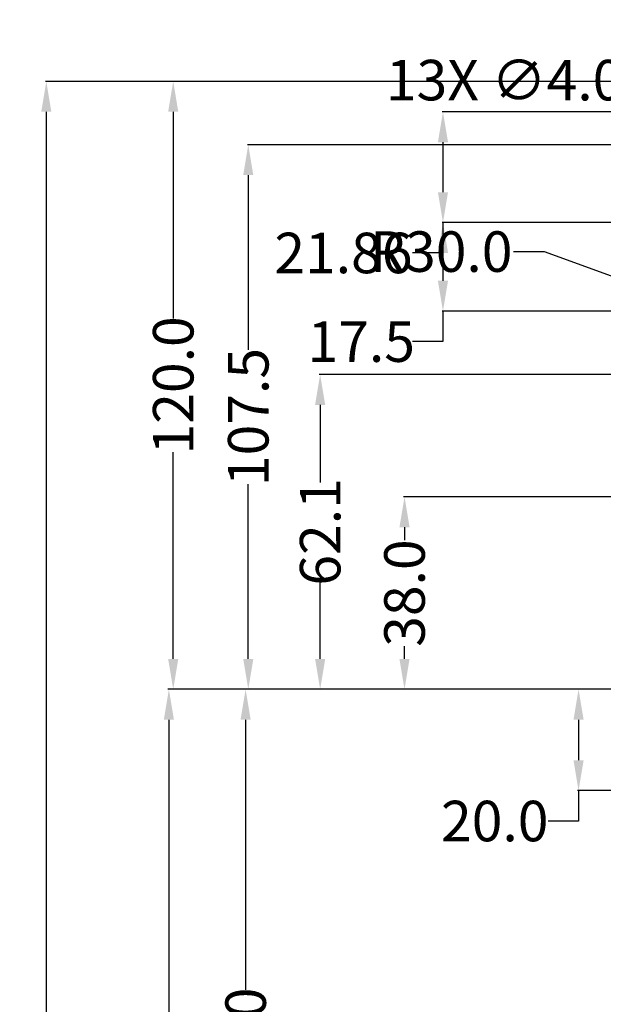
# Model space of a CAD drawing. Units: inches. Extents: x 11765 to 12471, y 10149 to 10793.
# Tile 3 of 8: x 11765 to 11880, y 10530 to 10724. Entities that reach past the tile are written whole.
import ezdxf

# ---------------------------------------------------------------- set-up
doc = ezdxf.new("R2010")
doc.units = ezdxf.units.IN
doc.header["$MEASUREMENT"] = 0
doc.layers.add('M-DIMS', color=2, linetype='Continuous', lineweight=25)
doc.styles.get("Standard").update_dxf_attribs({"font": 'arial.ttf'})
doc.dimstyles.get("Standard").update_dxf_attribs({"dimtxt": 8, "dimasz": 6, "dimexe": 0.18, "dimexo": 0.0625, "dimgap": 0.09, "dimtad": 0, "dimtoh": 1, "dimdec": 1, "dimzin": 0, "dimdsep": 46, "dimtxsty": 'Standard', "dimcen": 0.09, "dimadec": 0, "dimazin": 0, "dimtfac": 1, "dimtdec": 1, "dimtofl": 0, "dimtmove": 0, "dimatfit": 3, "dimfxl": 1, "dimtolj": 1, "dimtzin": 0, "dimarcsym": 0})

# ---------------------------------------------------------------- blocks, each defined once
blk = doc.blocks.new('*D6')
at = {"layer": 'Defpoints', "color": 0, "transparency": 16777216}
for p in [(11882.91, 10712.15), (11769.87, 10237.15), (11917.55, 10237.15)]:
    blk.add_point(p, dxfattribs=at)
at = {"layer": 'M-DIMS', "color": 0, "lineweight": -2, "transparency": 16777216}
for p, q in [((11882.85, 10712.15), (11769.69, 10712.15)), ((11769.87, 10706.15), (11769.87, 10488.38)), ((11769.87, 10243.15), (11769.87, 10460.91)), ((11917.49, 10237.15), (11769.69, 10237.15))]:
    blk.add_line(p, q, dxfattribs=at)
at = {"layer": 'M-DIMS', "color": 0, "transparency": 16777216}
for points in [[(11768.87, 10706.15), (11770.87, 10706.15), (11769.87, 10712.15)], [(11768.87, 10243.15), (11770.87, 10243.15), (11769.87, 10237.15)]]:
    blk.add_solid(points, dxfattribs=at)
at = {"layer": 'M-DIMS', "color": 0, "transparency": 16777216, "insert": (11769.87, 10474.65), "char_height": 8, "attachment_point": 5, "rotation": 90}
blk.add_mtext('\\A1;475.0', dxfattribs=at)
blk = doc.blocks.new('*D24')
at = {"layer": 'Defpoints', "color": 0, "transparency": 16777216}
for p in [(11794.92, 10712.15), (11882.91, 10712.15), (11882.91, 10592.15)]:
    blk.add_point(p, dxfattribs=at)
at = {"layer": 'M-DIMS', "color": 0, "lineweight": -2, "transparency": 16777216}
for p, q in [((11882.85, 10712.15), (11794.74, 10712.15)), ((11794.92, 10706.15), (11794.92, 10665.34)), ((11794.92, 10598.15), (11794.92, 10638.95)), ((11882.85, 10592.15), (11794.74, 10592.15))]:
    blk.add_line(p, q, dxfattribs=at)
at = {"layer": 'M-DIMS', "color": 0, "transparency": 16777216}
for points in [[(11793.92, 10706.15), (11795.92, 10706.15), (11794.92, 10712.15)], [(11793.92, 10598.15), (11795.92, 10598.15), (11794.92, 10592.15)]]:
    blk.add_solid(points, dxfattribs=at)
at = {"layer": 'M-DIMS', "color": 0, "transparency": 16777216, "insert": (11794.92, 10652.15), "char_height": 8, "attachment_point": 5, "rotation": 90}
blk.add_mtext('\\A1;120.0', dxfattribs=at)
blk = doc.blocks.new('*D25')
at = {"layer": 'Defpoints', "color": 0, "transparency": 16777216}
for p in [(11894.91, 10699.65), (11809.73, 10592.15), (11882.91, 10592.15)]:
    blk.add_point(p, dxfattribs=at)
at = {"layer": 'M-DIMS', "color": 0, "lineweight": -2, "transparency": 16777216}
for p, q in [((11894.85, 10699.65), (11809.55, 10699.65)), ((11809.73, 10693.65), (11809.73, 10659.14)), ((11809.73, 10598.15), (11809.73, 10632.65)), ((11882.85, 10592.15), (11809.55, 10592.15))]:
    blk.add_line(p, q, dxfattribs=at)
at = {"layer": 'M-DIMS', "color": 0, "transparency": 16777216}
for points in [[(11808.73, 10693.65), (11810.73, 10693.65), (11809.73, 10699.65)], [(11808.73, 10598.15), (11810.73, 10598.15), (11809.73, 10592.15)]]:
    blk.add_solid(points, dxfattribs=at)
at = {"layer": 'M-DIMS', "color": 0, "transparency": 16777216, "insert": (11809.73, 10645.9), "char_height": 8, "attachment_point": 5, "rotation": 90}
blk.add_mtext('\\A1;107.5', dxfattribs=at)
blk = doc.blocks.new('*D26')
at = {"layer": 'Defpoints', "color": 0, "transparency": 16777216}
for p in [(11934.91, 10654.29), (11823.92, 10592.15), (11882.91, 10592.15)]:
    blk.add_point(p, dxfattribs=at)
at = {"layer": 'M-DIMS', "color": 0, "lineweight": -2, "transparency": 16777216}
for p, q in [((11934.85, 10654.29), (11823.74, 10654.29)), ((11823.92, 10648.29), (11823.92, 10632.95)), ((11823.92, 10598.15), (11823.92, 10613.49)), ((11882.85, 10592.15), (11823.74, 10592.15))]:
    blk.add_line(p, q, dxfattribs=at)
at = {"layer": 'M-DIMS', "color": 0, "transparency": 16777216}
for points in [[(11822.92, 10648.29), (11824.92, 10648.29), (11823.92, 10654.29)], [(11822.92, 10598.15), (11824.92, 10598.15), (11823.92, 10592.15)]]:
    blk.add_solid(points, dxfattribs=at)
at = {"layer": 'M-DIMS', "color": 0, "transparency": 16777216, "insert": (11823.92, 10623.22), "char_height": 8, "attachment_point": 5, "rotation": 90}
blk.add_mtext('\\A1;62.1', dxfattribs=at)
blk = doc.blocks.new('*D27')
at = {"layer": 'Defpoints', "color": 0, "transparency": 16777216}
for p in [(11840.57, 10630.15), (11942.91, 10630.15), (11942.91, 10592.15)]:
    blk.add_point(p, dxfattribs=at)
at = {"layer": 'M-DIMS', "color": 0, "lineweight": -2, "transparency": 16777216}
for p, q in [((11942.85, 10630.15), (11840.39, 10630.15)), ((11840.57, 10624.15), (11840.57, 10621.61)), ((11840.57, 10598.15), (11840.57, 10600.68)), ((11942.85, 10592.15), (11840.39, 10592.15))]:
    blk.add_line(p, q, dxfattribs=at)
at = {"layer": 'M-DIMS', "color": 0, "transparency": 16777216}
for points in [[(11839.57, 10624.15), (11841.57, 10624.15), (11840.57, 10630.15)], [(11839.57, 10598.15), (11841.57, 10598.15), (11840.57, 10592.15)]]:
    blk.add_solid(points, dxfattribs=at)
at = {"layer": 'M-DIMS', "color": 0, "transparency": 16777216, "insert": (11840.57, 10611.15), "char_height": 8, "attachment_point": 5, "rotation": 90}
blk.add_mtext('\\A1;38.0', dxfattribs=at)
blk = doc.blocks.new('*D29')
at = {"layer": 'Defpoints', "color": 0, "transparency": 16777216}
for p in [(11794.06, 10592.15), (11889.16, 10592.15), (11894.91, 10322.15)]:
    blk.add_point(p, dxfattribs=at)
at = {"layer": 'M-DIMS', "color": 0, "lineweight": -2, "transparency": 16777216}
for p, q in [((11889.1, 10592.15), (11793.88, 10592.15)), ((11794.06, 10586.15), (11794.06, 10470.79)), ((11794.06, 10328.15), (11794.06, 10443.5)), ((11894.85, 10322.15), (11793.88, 10322.15))]:
    blk.add_line(p, q, dxfattribs=at)
at = {"layer": 'M-DIMS', "color": 0, "transparency": 16777216}
for points in [[(11793.06, 10586.15), (11795.06, 10586.15), (11794.06, 10592.15)], [(11793.06, 10328.15), (11795.06, 10328.15), (11794.06, 10322.15)]]:
    blk.add_solid(points, dxfattribs=at)
at = {"layer": 'M-DIMS', "color": 0, "transparency": 16777216, "insert": (11794.06, 10457.15), "char_height": 8, "attachment_point": 5, "rotation": 90}
blk.add_mtext('\\A1;270.0', dxfattribs=at)
blk = doc.blocks.new('*D30')
at = {"layer": 'Defpoints', "color": 0, "transparency": 16777216}
for p in [(11872.35, 10592.15), (11809.21, 10447.15), (11894.91, 10447.15)]:
    blk.add_point(p, dxfattribs=at)
at = {"layer": 'M-DIMS', "color": 0, "lineweight": -2, "transparency": 16777216}
for p, q in [((11872.29, 10592.15), (11809.03, 10592.15)), ((11809.21, 10586.15), (11809.21, 10532.84)), ((11809.21, 10453.15), (11809.21, 10506.45)), ((11894.85, 10447.15), (11809.03, 10447.15))]:
    blk.add_line(p, q, dxfattribs=at)
at = {"layer": 'M-DIMS', "color": 0, "transparency": 16777216}
for points in [[(11808.21, 10586.15), (11810.21, 10586.15), (11809.21, 10592.15)], [(11808.21, 10453.15), (11810.21, 10453.15), (11809.21, 10447.15)]]:
    blk.add_solid(points, dxfattribs=at)
at = {"layer": 'M-DIMS', "color": 0, "transparency": 16777216, "insert": (11809.21, 10519.65), "char_height": 8, "attachment_point": 5, "rotation": 90}
blk.add_mtext('\\A1;145.0', dxfattribs=at)
blk = doc.blocks.new('*D31')
at = {"layer": 'Defpoints', "color": 0, "transparency": 16777216}
for p in [(11895.41, 10592.15), (11874.92, 10572.15), (11894.91, 10572.15)]:
    blk.add_point(p, dxfattribs=at)
at = {"layer": 'M-DIMS', "color": 0, "lineweight": -2, "transparency": 16777216}
for p, q in [((11895.35, 10592.15), (11874.74, 10592.15)), ((11874.92, 10586.15), (11874.92, 10578.15)), ((11894.85, 10572.15), (11874.74, 10572.15)), ((11874.92, 10572.15), (11874.92, 10566.15)), ((11874.92, 10566.15), (11868.92, 10566.15))]:
    blk.add_line(p, q, dxfattribs=at)
at = {"layer": 'M-DIMS', "color": 0, "transparency": 16777216}
for points in [[(11873.92, 10586.15), (11875.92, 10586.15), (11874.92, 10592.15)], [(11873.92, 10578.15), (11875.92, 10578.15), (11874.92, 10572.15)]]:
    blk.add_solid(points, dxfattribs=at)
at = {"layer": 'M-DIMS', "color": 0, "transparency": 16777216, "insert": (11858.38, 10566.15), "char_height": 8, "attachment_point": 5}
blk.add_mtext('\\A1;20.0', dxfattribs=at)
blk = doc.blocks.new('*D35')
at = {"layer": 'Defpoints', "color": 0, "transparency": 16777216}
for p in [(11906.72, 10664.53), (11934.91, 10654.29)]:
    blk.add_point(p, dxfattribs=at)
at = {"layer": 'M-DIMS', "color": 0, "lineweight": -2, "transparency": 16777216}
for p, q in [((11862.11, 10678.56), (11868.11, 10678.56)), ((11868.11, 10678.56), (11901.08, 10666.58)), ((11934.82, 10654.29), (11935, 10654.29)), ((11934.91, 10654.2), (11934.91, 10654.38))]:
    blk.add_line(p, q, dxfattribs=at)
at = {"layer": 'M-DIMS', "color": 0, "transparency": 16777216}
blk.add_solid([(11901.42, 10667.52), (11900.74, 10665.64), (11906.72, 10664.53)], dxfattribs=at)
at = {"layer": 'M-DIMS', "color": 0, "transparency": 16777216, "insert": (11847.81, 10678.56), "char_height": 8, "attachment_point": 5}
blk.add_mtext('\\A1;R30.0', dxfattribs=at)
blk = doc.blocks.new('*D62')
at = {"layer": 'Defpoints', "color": 0, "transparency": 16777216}
for p in [(12379.9, 10706.15), (11848.16, 10684.29), (12385.4, 10684.29)]:
    blk.add_point(p, dxfattribs=at)
at = {"layer": 'M-DIMS', "color": 0, "lineweight": -2, "transparency": 16777216}
for p, q in [((12379.83, 10706.15), (11847.98, 10706.15)), ((11848.16, 10700.15), (11848.16, 10690.29)), ((12385.33, 10684.29), (11847.98, 10684.29)), ((11848.16, 10684.29), (11848.16, 10678.29)), ((11848.16, 10678.29), (11842.16, 10678.29))]:
    blk.add_line(p, q, dxfattribs=at)
at = {"layer": 'M-DIMS', "color": 0, "transparency": 16777216}
for points in [[(11847.16, 10700.15), (11849.16, 10700.15), (11848.16, 10706.15)], [(11847.16, 10690.29), (11849.16, 10690.29), (11848.16, 10684.29)]]:
    blk.add_solid(points, dxfattribs=at)
at = {"layer": 'M-DIMS', "color": 0, "transparency": 16777216, "insert": (11828.51, 10678.29), "char_height": 8, "attachment_point": 5}
blk.add_mtext('\\A1;21.86', dxfattribs=at)
blk = doc.blocks.new('*D63')
at = {"layer": 'Defpoints', "color": 0, "transparency": 16777216}
for p in [(12385.4, 10684.29), (11848.16, 10666.79), (12385.4, 10666.79)]:
    blk.add_point(p, dxfattribs=at)
at = {"layer": 'M-DIMS', "color": 0, "lineweight": -2, "transparency": 16777216}
for p, q in [((12385.33, 10684.29), (11847.98, 10684.29)), ((11848.16, 10678.29), (11848.16, 10672.79)), ((12385.33, 10666.79), (11847.98, 10666.79)), ((11848.16, 10666.79), (11848.16, 10660.79)), ((11848.16, 10660.79), (11842.16, 10660.79))]:
    blk.add_line(p, q, dxfattribs=at)
at = {"layer": 'M-DIMS', "color": 0, "transparency": 16777216}
for points in [[(11847.16, 10678.29), (11849.16, 10678.29), (11848.16, 10684.29)], [(11847.16, 10672.79), (11849.16, 10672.79), (11848.16, 10666.79)]]:
    blk.add_solid(points, dxfattribs=at)
at = {"layer": 'M-DIMS', "color": 0, "transparency": 16777216, "insert": (11832.03, 10660.79), "char_height": 8, "attachment_point": 5}
blk.add_mtext('\\A1;17.5', dxfattribs=at)
blk = doc.blocks.new('*D83')
at = {"layer": 'Defpoints', "color": 0, "transparency": 16777216}
for p in [(11894.09, 10701.47), (11895.73, 10697.82)]:
    blk.add_point(p, dxfattribs=at)
at = {"layer": 'M-DIMS', "color": 0, "lineweight": -2, "transparency": 16777216}
for p, q in [((11883.16, 10712.41), (11889.16, 10712.41)), ((11889.16, 10712.41), (11891.62, 10706.94)), ((11894.82, 10699.65), (11895, 10699.65)), ((11894.91, 10699.56), (11894.91, 10699.74))]:
    blk.add_line(p, q, dxfattribs=at)
at = {"layer": 'M-DIMS', "color": 0, "transparency": 16777216}
blk.add_solid([(11892.53, 10707.35), (11890.71, 10706.53), (11894.09, 10701.47)], dxfattribs=at)
at = {"layer": 'M-DIMS', "color": 0, "transparency": 16777216, "insert": (11860.33, 10712.41), "char_height": 8, "attachment_point": 5}
blk.add_mtext('\\A1;13X ∅4.0', dxfattribs=at)

msp = doc.modelspace()

# ---------------------------------------------------------------- dimensions: what is measured, and where the dimension line sits
at = {"layer": 'M-DIMS'}
dim = msp.add_diameter_dim_2p(p1=(11895.734, 10697.822), p2=(11894.09, 10701.469), text='13X <>', dimstyle='Standard', override={"dimdec": 1, "dimlfac": 1, "dimrnd": 0, "dimzin": 0, "dimdsep": 46, "dimlunit": 2}, dxfattribs=at)
dim.commit()
dim.dimension.update_dxf_attribs({"geometry": '*D83', "text_midpoint": (11860.332, 10712.407), "dimtype": 163})
for base, p1, p2, override, picture, middle in [((11769.869, 10237.146), (11882.912, 10712.146), (11917.553, 10237.146), {"dimclrd": 0, "dimclre": 0, "dimclrt": 0}, '*D6', (11769.869, 10474.646)), ((11794.917, 10712.146), (11882.912, 10592.146), (11882.912, 10712.146), {"dimclrd": 0, "dimclre": 0, "dimclrt": 0}, '*D24', (11794.917, 10652.146)), ((11848.162, 10684.286), (12379.896, 10706.146), (12385.396, 10684.286), {"dimdec": 2, "dimlfac": 1, "dimrnd": 0, "dimzin": 0, "dimdsep": 46, "dimlunit": 2}, '*D62', (11828.509, 10678.286)), ((11809.731, 10592.146), (11894.912, 10699.646), (11882.912, 10592.146), {"dimclrd": 0, "dimclre": 0, "dimclrt": 0}, '*D25', (11809.731, 10645.896)), ((11848.162, 10666.786), (12385.396, 10684.286), (12385.396, 10666.786), {"dimdec": 1, "dimlfac": 1, "dimrnd": 0, "dimzin": 0, "dimdsep": 46, "dimlunit": 2}, '*D63', (11832.028, 10660.786)), ((11823.918, 10592.146), (11934.912, 10654.286), (11882.912, 10592.146), {"dimclrd": 0, "dimclre": 0, "dimclrt": 0}, '*D26', (11823.918, 10623.216)), ((11840.567, 10630.146), (11942.912, 10592.146), (11942.912, 10630.146), {"dimclrd": 0, "dimclre": 0, "dimclrt": 0}, '*D27', (11840.567, 10611.146)), ((11794.063, 10592.146), (11894.912, 10322.146), (11889.162, 10592.146), {"dimclrd": 0, "dimclre": 0, "dimclrt": 0}, '*D29', (11794.063, 10457.146)), ((11809.207, 10447.146), (11872.348, 10592.146), (11894.912, 10447.146), {"dimclrd": 0, "dimclre": 0, "dimclrt": 0}, '*D30', (11809.207, 10519.646)), ((11874.915, 10572.146), (11895.412, 10592.146), (11894.912, 10572.146), {"dimclrd": 0, "dimclre": 0, "dimclrt": 0}, '*D31', (11858.381, 10566.146))]:
    dim = msp.add_linear_dim(base=base, p1=p1, p2=p2, angle=90, dimstyle='Standard', override=override, dxfattribs=at)
    dim.commit()
    dim.dimension.update_dxf_attribs({"geometry": picture, "text_midpoint": middle})
dim = msp.add_radius_dim(center=(11934.912, 10654.286), mpoint=(11906.716, 10664.533), dimstyle='Standard', override={"dimclrd": 0, "dimclre": 0, "dimclrt": 0}, dxfattribs=at)
dim.commit()
dim.dimension.update_dxf_attribs({"geometry": '*D35', "text_midpoint": (11847.813, 10678.564), "dimtype": 164})

doc.saveas('drawing.dxf')
